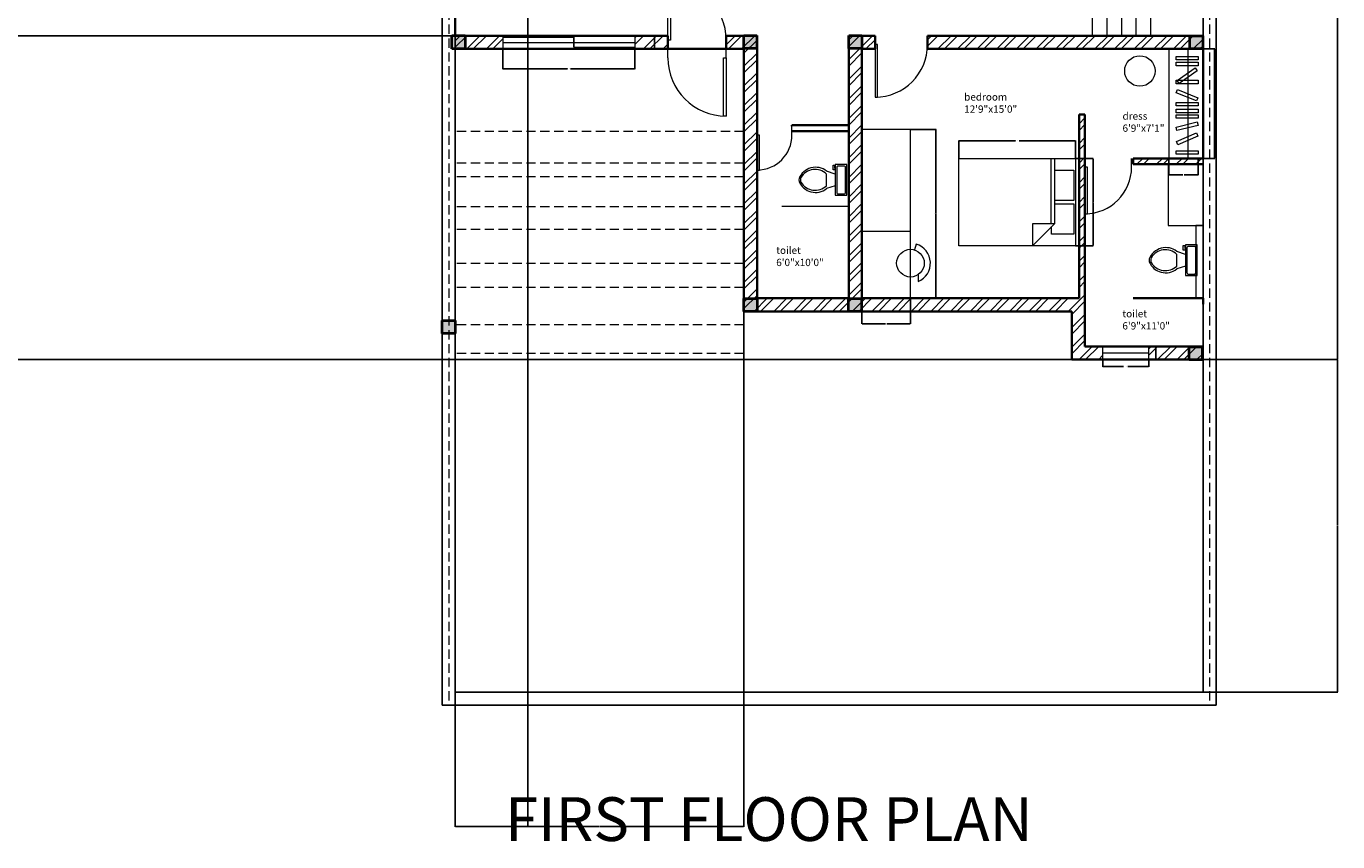
# Model space of a CAD drawing. Units: inches. Extents: x 19613 to 21413, y 12082 to 13202.
# Tile 7 of 9: x 20513 to 21413, y 12082 to 12641. Entities that reach past the tile are written whole.
import ezdxf

# ---------------------------------------------------------------- set-up
doc = ezdxf.new("R2010")
doc.units = ezdxf.units.IN
doc.linetypes.add('HIDDEN', pattern=[9.525, 6.35, -3.175])
for name, color, linetype, lineweight in [('A-ANNO-DIMS', 2, 'Continuous', 18), ('A-ANNO-TEXT', 7, 'Continuous', 30), ('A-AREA-IDEN', 7, 'Continuous', 18), ('A-COLS', 7, 'Continuous', 40), ('A-COLS-PATT', 6, 'Continuous', 13), ('A-DOOR', 3, 'Continuous', 18), ('A-FLOR-CASE', 9, 'Continuous', 18), ('A-FLOR-FIXT', 9, 'Continuous', 18), ('A-FLOR-HIDN', 8, 'HIDDEN', 13), ('A-FLOR-STRS', 7, 'Continuous', 18), ('A-FURN', 8, 'Continuous', 18), ('A-GLAZ', 4, 'Continuous', 18), ('A-WALL', 7, 'Continuous', 35), ('A-WALL-PATT', 252, 'Continuous', 13), ('C-PROP', 7, 'Continuous', 25), ('C-PROP-HIDN', 8, 'HIDDEN', 13)]:
    doc.layers.add(name, color=color, linetype=linetype, lineweight=lineweight)
doc.styles.get("Standard").update_dxf_attribs({"font": 'arial.ttf'})
doc.dimstyles.get("Standard").update_dxf_attribs({"dimtxt": 0.18, "dimasz": 0.18, "dimexe": 0.18, "dimexo": 0.0625, "dimgap": 0.09, "dimtad": 0, "dimtih": 1, "dimtoh": 1, "dimdec": 4, "dimzin": 0, "dimdsep": 46, "dimtxsty": 'Standard', "dimcen": 0.09, "dimadec": 0, "dimazin": 0, "dimtfac": 1, "dimtdec": 4, "dimtofl": 0, "dimtmove": 0, "dimatfit": 3, "dimfxl": 1, "dimtolj": 1, "dimtzin": 0, "dimarcsym": 0})

# ---------------------------------------------------------------- blocks, each defined once
blk = doc.blocks.new('Bed - Queen')
for p, q in [((0, -80.00003), (0, 0)), ((0, 0), (59.99999, 0)), ((59.99999, 0), (59.99999, -80.00003)), ((7.99999, -1.2), (28.79998, -1.2)), ((7.99999, -14.4), (7.99999, -1.2)), ((28.79998, -1.2), (28.79998, -14.4)), ((31.19999, -1.2), (51.99999, -1.2)), ((31.19999, -14.4), (31.19999, -1.2)), ((51.99999, -1.2), (51.99999, -16.4)), ((0, -14.4), (44.8, -14.4)), ((44.8, -16.8), (0, -16.8)), ((59.99999, -29.6), (44.8, -14.4)), ((44.8, -14.4), (44.8, -29.6)), ((51.99999, -16.4), (46.79936, -16.4)), ((44.8, -29.6), (59.99999, -29.6)), ((59.99999, -80.00003), (0, -80.00003))]:
    blk.add_line(p, q)
blk = doc.blocks.new('*U6')
for p, q in [((0, 0), (0, -6)), ((40, 0), (40, -6))]:
    blk.add_line(p, q)
blk.add_lwpolyline([(0, 0), (0, 40), (1.75, 40), (1.75, 0)], close=True)
blk.add_arc((0, 0), 40, 0, 90)
blk = doc.blocks.new('*U7')
for p, q in [((-40, 0), (-40, 6)), ((0, 0), (0, 6))]:
    blk.add_line(p, q)
blk.add_lwpolyline([(0, 0), (0, -40), (-1.75, -40), (-1.75, 0)], close=True)
blk.add_arc((0, 0), 40, 180, 270)
blk = doc.blocks.new('*U15')
for p, q in [((0, 0), (0, 6)), ((36, 0), (36, 6))]:
    blk.add_line(p, q)
blk.add_lwpolyline([(0, 0), (0, -36), (1.75, -36), (1.75, 0)], close=True)
blk.add_arc((0, 0), 36, 270, 0)
blk = doc.blocks.new('*U16')
for p, q in [((0, 0), (0, 6)), ((32, 0), (32, 6))]:
    blk.add_line(p, q)
blk.add_lwpolyline([(0, 0), (0, -32), (1.75, -32), (1.75, 0)], close=True)
blk.add_arc((0, 0), 32, 270, 0)
blk = doc.blocks.new('*U19')
for p, q in [((0, 0), (0, 6)), ((24, 0), (24, 6))]:
    blk.add_line(p, q)
blk.add_lwpolyline([(0, 0), (0, -24), (1.75, -24), (1.75, 0)], close=True)
blk.add_arc((0, 0), 24, 270, 0)
blk = doc.blocks.new('Toilet - top')
for p, q in [((-10, -8.5), (-8, -8.5)), ((-10, -9.5), (-10, -8.5)), ((-8, -8.5), (-8, -8)), ((-7, -8), (-7, -9.5)), ((-4, -8), (-6, -14)), ((4, -8), (6, -14)), ((9.5, -6), (9.5, -2)), ((-7, -9.5), (-10, -9.5)), ((4, -14), (-4, -14))]:
    blk.add_line(p, q)
blk.add_lwpolyline([(10.5, -8), (10.5, 0), (-10.5, 0), (-10.5, -8)], close=True)
for points in [[(-9.5, -2), (-9.5, -6)], [(8.5, -1), (-8.5, -1)], [(-8.5, -7), (8.5, -7)]]:
    blk.add_lwpolyline(points)
for centre, radius, start, end in [((-8.62, -1.88), 0.884, 81.8699, 188.1301), ((-8.62, -6.12), 0.884, 171.8699, 278.1301), ((8.62, -1.88), 0.884, 351.8699, 98.1301), ((8.62, -6.12), 0.884, 261.8699, 8.1301), ((3.52, -21.58), 12.17, 141.46911, 247.97143), ((4.2, -21.82), 11.33, 136.36773, 238.94682), ((-3.52, -21.58), 12.17, 292.02843, 38.53071), ((-4.2, -21.82), 11.33, 301.05301, 43.63209), ((0, -27.88), 4, 245.73182, 294.26817), ((0, -29), 4, 254.86053, 285.13947)]:
    blk.add_arc(centre, radius, start, end)
blk = doc.blocks.new('COL-9x9')
for p, q in [((0, 9), (9, 9)), ((0, 0), (0, 9)), ((9, 9), (9, 0)), ((9, 0), (0, 0))]:
    blk.add_line(p, q)
blk = doc.blocks.new('CLOSET-STRAIGHT-RAIL')
for p, q in [((0, 75), (0, 0)), ((12.99, 75), (12.99, 0))]:
    blk.add_line(p, q)
for points in [[(5.04, 69.91), (20.08, 69.91), (20.08, 67.47), (5.04, 67.47)], [(5.04, 65.98), (20.08, 65.98), (20.08, 63.54), (5.04, 63.54)], [(5.8, 53.4), (18.07, 62.1), (19.48, 60.12), (7.21, 51.41)], [(5.04, 53.51), (20.08, 53.51), (20.08, 51.08), (5.04, 51.08)], [(6.02, 47.16), (20, 41.61), (19.1, 39.35), (5.12, 44.9)], [(5.04, 38.4), (20.08, 38.4), (20.08, 35.96), (5.04, 35.96)], [(5.04, 33.62), (20.08, 33.62), (20.08, 31.19), (5.04, 31.19)], [(5.04, 29.93), (20.08, 29.93), (20.08, 27.49), (5.04, 27.49)], [(4.97, 21.36), (19.58, 24.94), (20.16, 22.57), (5.55, 18.99)], [(5.22, 11.51), (19.01, 17.5), (19.98, 15.27), (6.19, 9.28)], [(5.04, 5.23), (20.08, 5.23), (20.08, 2.79), (5.04, 2.79)]]:
    blk.add_lwpolyline(points, close=True)
blk = doc.blocks.new('WINDOW-LIVING-SLIDER')
for p, q in [((0, 9), (0, 0)), ((90.49, 9), (90.49, 0)), ((0, 8.08), (48.53, 8.08)), ((0, 4.5), (48.53, 4.5)), ((48.53, 4.5), (48.53, 8.08)), ((48.53, 8.08), (48.53, 1.28)), ((48.53, 1.28), (48.53, 4.5)), ((48.53, 4.5), (90.49, 4.5)), ((48.53, 1.28), (90.49, 1.28)), ((90.49, 6.86), (90.49, 4.5))]:
    blk.add_line(p, q)
blk = doc.blocks.new('WINDOW-BATH')
for p, q in [((0, 9), (0, 0)), ((31.63, 9), (31.63, 0)), ((0, 4.5), (31.63, 4.5))]:
    blk.add_line(p, q)
blk = doc.blocks.new('DESK-CHAIR-ROUND-LARGE')
for p, q in [((13.49, 25.67), (12.27, 21.68)), ((14.77, 4.71), (14.81, 0))]:
    blk.add_line(p, q)
blk.add_circle((9.49, 12.6), 9.49)
blk.add_circle((9.49, 12.6), 9.49)
blk.add_arc((9.49, 12.6), 13.67, 292.8714, 73.00761)
blk = doc.blocks.new('BEDROOM-DESK-WIDE')
for p, q in [((33.29, 115.88), (0, 115.88)), ((33.29, 0), (33.29, 115.88)), ((33.29, 45.86), (0, 45.86)), ((0, 0), (0, 0)), ((0, 0), (33.29, 0))]:
    blk.add_line(p, q)
blk = doc.blocks.new('STAIR-RETURN-FLIGHT')
for p, q in [((0, 169), (0, 133)), ((10, 169), (10, 133)), ((20, 169), (20, 133)), ((30, 169), (30, 133)), ((76, 169), (40, 169)), ((76, 169), (40, 169)), ((40, 169), (40, 0)), ((76, 169), (76, 133)), ((76, 169), (76, 133)), ((76, 133), (0, 133)), ((76, 123), (40, 123)), ((76, 113), (40, 113)), ((76, 103), (40, 103)), ((76, 93), (40, 93)), ((76, 83), (40, 83)), ((76, 73), (40, 73)), ((76, 63), (40, 63)), ((76, 31), (76, 67)), ((76, 53), (40, 53)), ((76, 36), (0, 36)), ((0, 36), (0, 0)), ((10, 36), (10, 0)), ((20, 36), (20, 0)), ((30, 36), (30, 0)), ((76, 43), (40, 43)), ((76, 0), (76, 36))]:
    blk.add_line(p, q)
blk = doc.blocks.new('*D41')
at = {"layer": 'A-ANNO-DIMS', "color": 0, "lineweight": -2, "transparency": 16777216}
for p, q in [((21153, 12550.29), (21153, 12562.41)), ((21153.18, 12562.23), (21191.69, 12562.23)), ((21232.82, 12562.23), (21194.3, 12562.23)), ((21233, 12550.29), (21233, 12562.41))]:
    blk.add_line(p, q, dxfattribs=at)
at = {"layer": 'A-ANNO-DIMS', "color": 0, "transparency": 16777216}
for points in [[(21153.18, 12562.26), (21153.18, 12562.2), (21153, 12562.23)], [(21232.82, 12562.26), (21232.82, 12562.2), (21233, 12562.23)]]:
    blk.add_solid(points, dxfattribs=at)
at = {"layer": 'Defpoints', "color": 0, "transparency": 16777216}
for p in [(21233, 12562.23), (21153, 12550.23), (21233, 12550.23)]:
    blk.add_point(p, dxfattribs=at)
at = {"layer": 'A-ANNO-DIMS', "color": 0, "transparency": 16777216, "insert": (21193, 12562.23), "char_height": 0.18, "attachment_point": 5}
blk.add_mtext('\\A1;QUEEN BED 80 TYP.', dxfattribs=at)
blk = doc.blocks.new('*D42')
at = {"layer": 'A-ANNO-DIMS', "color": 0, "lineweight": -2, "transparency": 16777216}
for p, q in [((21233.06, 12550.23), (21245.18, 12550.23)), ((21245, 12550.05), (21245, 12520.41)), ((21245, 12490.41), (21245, 12520.05)), ((21233.06, 12490.23), (21245.18, 12490.23))]:
    blk.add_line(p, q, dxfattribs=at)
at = {"layer": 'A-ANNO-DIMS', "color": 0, "transparency": 16777216}
for points in [[(21244.97, 12550.05), (21245.03, 12550.05), (21245, 12550.23)], [(21244.97, 12490.41), (21245.03, 12490.41), (21245, 12490.23)]]:
    blk.add_solid(points, dxfattribs=at)
at = {"layer": 'Defpoints', "color": 0, "transparency": 16777216}
for p in [(21233, 12550.23), (21233, 12490.23), (21245, 12490.23)]:
    blk.add_point(p, dxfattribs=at)
at = {"layer": 'A-ANNO-DIMS', "color": 0, "transparency": 16777216, "insert": (21245, 12520.23), "char_height": 0.18, "attachment_point": 5}
blk.add_mtext('\\A1;60 TYP.', dxfattribs=at)
blk = doc.blocks.new('*D57')
at = {"layer": 'A-ANNO-DIMS', "color": 0, "lineweight": -2, "transparency": 16777216}
for p, q in [((21317.16, 12625.28), (21328.52, 12625.28)), ((21328.34, 12625.1), (21328.34, 12587.96)), ((21328.34, 12550.46), (21328.34, 12587.6)), ((21317.16, 12550.28), (21328.52, 12550.28))]:
    blk.add_line(p, q, dxfattribs=at)
at = {"layer": 'A-ANNO-DIMS', "color": 0, "transparency": 16777216}
for points in [[(21328.31, 12625.1), (21328.37, 12625.1), (21328.34, 12625.28)], [(21328.31, 12550.46), (21328.37, 12550.46), (21328.34, 12550.28)]]:
    blk.add_solid(points, dxfattribs=at)
at = {"layer": 'Defpoints', "color": 0, "transparency": 16777216}
for p in [(21317.09, 12625.28), (21328.34, 12625.28), (21317.09, 12550.28)]:
    blk.add_point(p, dxfattribs=at)
at = {"layer": 'A-ANNO-DIMS', "color": 0, "transparency": 16777216, "insert": (21328.34, 12587.78), "char_height": 0.18, "attachment_point": 5}
blk.add_mtext('\\A1;RAIL 75 TYP.', dxfattribs=at)
blk = doc.blocks.new('*D58')
at = {"layer": 'A-ANNO-DIMS', "color": 0, "lineweight": -2, "transparency": 16777216}
for p, q in [((21296.94, 12550.22), (21296.94, 12538.85)), ((21317.09, 12550.22), (21317.09, 12538.85)), ((21297.12, 12539.03), (21306.49, 12539.03)), ((21316.91, 12539.03), (21307.55, 12539.03))]:
    blk.add_line(p, q, dxfattribs=at)
at = {"layer": 'A-ANNO-DIMS', "color": 0, "transparency": 16777216}
for points in [[(21297.12, 12539.06), (21297.12, 12539), (21296.94, 12539.03)], [(21316.91, 12539.06), (21316.91, 12539), (21317.09, 12539.03)]]:
    blk.add_solid(points, dxfattribs=at)
at = {"layer": 'Defpoints', "color": 0, "transparency": 16777216}
for p in [(21296.94, 12550.28), (21317.09, 12550.28), (21317.09, 12539.03)]:
    blk.add_point(p, dxfattribs=at)
at = {"layer": 'A-ANNO-DIMS', "color": 0, "transparency": 16777216, "insert": (21307.02, 12539.03), "char_height": 0.18, "attachment_point": 5}
blk.add_mtext('\\A1;20 TYP.', dxfattribs=at)
blk = doc.blocks.new('*D59')
at = {"layer": 'A-ANNO-DIMS', "color": 0, "lineweight": -2, "transparency": 16777216}
for p, q in [((20840.13, 12625.22), (20840.13, 12611.53)), ((20930.62, 12625.22), (20930.62, 12611.53)), ((20840.31, 12611.71), (20884.36, 12611.71)), ((20930.44, 12611.71), (20886.39, 12611.71))]:
    blk.add_line(p, q, dxfattribs=at)
at = {"layer": 'A-ANNO-DIMS', "color": 0, "transparency": 16777216}
for points in [[(20840.31, 12611.74), (20840.31, 12611.68), (20840.13, 12611.71)], [(20930.44, 12611.74), (20930.44, 12611.68), (20930.62, 12611.71)]]:
    blk.add_solid(points, dxfattribs=at)
at = {"layer": 'Defpoints', "color": 0, "transparency": 16777216}
for p in [(20840.13, 12625.28), (20930.62, 12625.28), (20930.62, 12611.71)]:
    blk.add_point(p, dxfattribs=at)
at = {"layer": 'A-ANNO-DIMS', "color": 0, "transparency": 16777216, "insert": (20885.38, 12611.71), "char_height": 0.18, "attachment_point": 5}
blk.add_mtext('\\A1;SLIDER 90 TYP.', dxfattribs=at)
blk = doc.blocks.new('*D60')
at = {"layer": 'A-ANNO-DIMS', "color": 0, "lineweight": -2, "transparency": 16777216}
for p, q in [((20930.68, 12634.28), (20944.37, 12634.28)), ((20944.19, 12634.1), (20944.19, 12629.96)), ((20930.68, 12625.28), (20944.37, 12625.28)), ((20944.19, 12625.46), (20944.19, 12629.6))]:
    blk.add_line(p, q, dxfattribs=at)
at = {"layer": 'A-ANNO-DIMS', "color": 0, "transparency": 16777216}
for points in [[(20944.16, 12634.1), (20944.22, 12634.1), (20944.19, 12634.28)], [(20944.16, 12625.46), (20944.22, 12625.46), (20944.19, 12625.28)]]:
    blk.add_solid(points, dxfattribs=at)
at = {"layer": 'Defpoints', "color": 0, "transparency": 16777216}
for p in [(20930.62, 12634.28), (20944.19, 12634.28), (20930.62, 12625.28)]:
    blk.add_point(p, dxfattribs=at)
at = {"layer": 'A-ANNO-DIMS', "color": 0, "transparency": 16777216, "insert": (20944.19, 12629.78), "char_height": 0.18, "attachment_point": 5}
blk.add_mtext('\\A1;9 TYP.', dxfattribs=at)
blk = doc.blocks.new('*D69')
at = {"layer": 'A-ANNO-DIMS', "color": 0, "lineweight": -2, "transparency": 16777216}
for p, q in [((21251.59, 12412.22), (21251.59, 12407.35)), ((21283.22, 12412.22), (21283.22, 12407.35)), ((21251.77, 12407.53), (21265.92, 12407.53)), ((21283.04, 12407.53), (21268.89, 12407.53))]:
    blk.add_line(p, q, dxfattribs=at)
at = {"layer": 'A-ANNO-DIMS', "color": 0, "transparency": 16777216}
for points in [[(21251.77, 12407.56), (21251.77, 12407.5), (21251.59, 12407.53)], [(21283.04, 12407.56), (21283.04, 12407.5), (21283.22, 12407.53)]]:
    blk.add_solid(points, dxfattribs=at)
at = {"layer": 'Defpoints', "color": 0, "transparency": 16777216}
for p in [(21251.59, 12412.28), (21283.22, 12412.28), (21251.59, 12407.53)]:
    blk.add_point(p, dxfattribs=at)
at = {"layer": 'A-ANNO-DIMS', "color": 0, "transparency": 16777216, "insert": (21267.41, 12407.53), "char_height": 0.18, "attachment_point": 5}
blk.add_mtext('\\A1;BATH WINDOW 32 TYP.', dxfattribs=at)
blk = doc.blocks.new('*D70')
at = {"layer": 'A-ANNO-DIMS', "color": 0, "lineweight": -2, "transparency": 16777216}
for p, q in [((21283.28, 12421.28), (21288.15, 12421.28)), ((21287.97, 12421.1), (21287.97, 12416.96)), ((21283.28, 12412.28), (21288.15, 12412.28)), ((21287.97, 12412.46), (21287.97, 12416.6))]:
    blk.add_line(p, q, dxfattribs=at)
at = {"layer": 'A-ANNO-DIMS', "color": 0, "transparency": 16777216}
for points in [[(21287.94, 12421.1), (21288, 12421.1), (21287.97, 12421.28)], [(21287.94, 12412.46), (21288, 12412.46), (21287.97, 12412.28)]]:
    blk.add_solid(points, dxfattribs=at)
at = {"layer": 'Defpoints', "color": 0, "transparency": 16777216}
for p in [(21283.22, 12421.28), (21283.22, 12412.28), (21287.97, 12412.28)]:
    blk.add_point(p, dxfattribs=at)
at = {"layer": 'A-ANNO-DIMS', "color": 0, "transparency": 16777216, "insert": (21287.97, 12416.78), "char_height": 0.18, "attachment_point": 5}
blk.add_mtext('\\A1;9 TYP.', dxfattribs=at)
blk = doc.blocks.new('*D73')
at = {"layer": 'A-ANNO-DIMS', "color": 0, "lineweight": -2, "transparency": 16777216}
for p, q in [((21119.79, 12570.15), (21137.29, 12570.15)), ((21137.11, 12569.97), (21137.11, 12512.4)), ((21137.11, 12454.46), (21137.11, 12512.03)), ((21119.79, 12454.28), (21137.29, 12454.28))]:
    blk.add_line(p, q, dxfattribs=at)
at = {"layer": 'A-ANNO-DIMS', "color": 0, "transparency": 16777216}
for points in [[(21137.08, 12569.97), (21137.14, 12569.97), (21137.11, 12570.15)], [(21137.08, 12454.46), (21137.14, 12454.46), (21137.11, 12454.28)]]:
    blk.add_solid(points, dxfattribs=at)
at = {"layer": 'Defpoints', "color": 0, "transparency": 16777216}
for p in [(21119.73, 12570.15), (21137.11, 12570.15), (21119.73, 12454.28)]:
    blk.add_point(p, dxfattribs=at)
at = {"layer": 'A-ANNO-DIMS', "color": 0, "transparency": 16777216, "insert": (21137.11, 12512.22), "char_height": 0.18, "attachment_point": 5}
blk.add_mtext('\\A1;DESK 116 TYP.', dxfattribs=at)
blk = doc.blocks.new('*D74')
at = {"layer": 'A-ANNO-DIMS', "color": 0, "lineweight": -2, "transparency": 16777216}
for p, q in [((21086.43, 12454.22), (21086.43, 12436.72)), ((21119.73, 12454.22), (21119.73, 12436.72)), ((21086.61, 12436.9), (21102.55, 12436.9)), ((21119.55, 12436.9), (21103.61, 12436.9))]:
    blk.add_line(p, q, dxfattribs=at)
at = {"layer": 'A-ANNO-DIMS', "color": 0, "transparency": 16777216}
for points in [[(21086.61, 12436.93), (21086.61, 12436.87), (21086.43, 12436.9)], [(21119.55, 12436.93), (21119.55, 12436.87), (21119.73, 12436.9)]]:
    blk.add_solid(points, dxfattribs=at)
at = {"layer": 'Defpoints', "color": 0, "transparency": 16777216}
for p in [(21086.43, 12454.28), (21119.73, 12454.28), (21119.73, 12436.9)]:
    blk.add_point(p, dxfattribs=at)
at = {"layer": 'A-ANNO-DIMS', "color": 0, "transparency": 16777216, "insert": (21103.08, 12436.9), "char_height": 0.18, "attachment_point": 5}
blk.add_mtext('\\A1;33 TYP.', dxfattribs=at)
blk = doc.blocks.new('*D87')
at = {"layer": 'A-ANNO-DIMS', "color": 0, "lineweight": -2, "transparency": 16777216}
for p, q in [((20218.76, 12982.28), (21412.86, 12982.28)), ((21412.68, 12982.1), (21412.68, 12697.46)), ((21412.68, 12412.46), (21412.68, 12697.1)), ((20218.76, 12412.28), (21412.86, 12412.28))]:
    blk.add_line(p, q, dxfattribs=at)
at = {"layer": 'A-ANNO-DIMS', "color": 0, "transparency": 16777216}
for points in [[(21412.65, 12982.1), (21412.71, 12982.1), (21412.68, 12982.28)], [(21412.65, 12412.46), (21412.71, 12412.46), (21412.68, 12412.28)]]:
    blk.add_solid(points, dxfattribs=at)
at = {"layer": 'Defpoints', "color": 0, "transparency": 16777216}
for p in [(20218.69, 12982.28), (21412.68, 12982.28), (20218.69, 12412.28)]:
    blk.add_point(p, dxfattribs=at)
at = {"layer": 'A-ANNO-DIMS', "color": 0, "transparency": 16777216, "insert": (21412.68, 12697.28), "char_height": 0.18, "attachment_point": 5}
blk.add_mtext('\\A1;570', dxfattribs=at)
blk = doc.blocks.new('*D88')
at = {"layer": 'A-ANNO-DIMS', "color": 0, "lineweight": -2, "transparency": 16777216}
for p, q in [((21320.5, 12412.28), (21412.86, 12412.28)), ((21412.68, 12412.1), (21412.68, 12298.46)), ((21412.68, 12184.46), (21412.68, 12298.1)), ((21320.5, 12184.28), (21412.86, 12184.28))]:
    blk.add_line(p, q, dxfattribs=at)
at = {"layer": 'A-ANNO-DIMS', "color": 0, "transparency": 16777216}
for points in [[(21412.65, 12412.1), (21412.71, 12412.1), (21412.68, 12412.28)], [(21412.65, 12184.46), (21412.71, 12184.46), (21412.68, 12184.28)]]:
    blk.add_solid(points, dxfattribs=at)
at = {"layer": 'Defpoints', "color": 0, "transparency": 16777216}
for p in [(21320.43, 12412.28), (21412.68, 12412.28), (21320.43, 12184.28)]:
    blk.add_point(p, dxfattribs=at)
at = {"layer": 'A-ANNO-DIMS', "color": 0, "transparency": 16777216, "insert": (21412.68, 12298.28), "char_height": 0.18, "attachment_point": 5}
blk.add_mtext('\\A1;228', dxfattribs=at)
blk = doc.blocks.new('*D89')
at = {"layer": 'A-ANNO-DIMS', "color": 0, "lineweight": -2, "transparency": 16777216}
for p, q in [((20807.37, 12808.28), (19613.26, 12808.28)), ((19613.44, 12808.1), (19613.44, 12721.46)), ((19613.44, 12634.46), (19613.44, 12721.1)), ((20807.37, 12634.28), (19613.26, 12634.28))]:
    blk.add_line(p, q, dxfattribs=at)
at = {"layer": 'A-ANNO-DIMS', "color": 0, "transparency": 16777216}
for points in [[(19613.41, 12808.1), (19613.47, 12808.1), (19613.44, 12808.28)], [(19613.41, 12634.46), (19613.47, 12634.46), (19613.44, 12634.28)]]:
    blk.add_solid(points, dxfattribs=at)
at = {"layer": 'Defpoints', "color": 0, "transparency": 16777216}
for p in [(19613.44, 12808.28), (20807.43, 12808.28), (20807.43, 12634.28)]:
    blk.add_point(p, dxfattribs=at)
at = {"layer": 'A-ANNO-DIMS', "color": 0, "transparency": 16777216, "insert": (19613.44, 12721.28), "char_height": 0.18, "attachment_point": 5}
blk.add_mtext('\\A1;174', dxfattribs=at)
blk = doc.blocks.new('*D99')
at = {"layer": 'A-ANNO-DIMS', "color": 0, "lineweight": -2, "transparency": 16777216}
for p, q in [((21320.5, 12982.28), (21412.86, 12982.28)), ((21412.68, 12982.1), (21412.68, 12697.46)), ((21412.68, 12412.46), (21412.68, 12697.1)), ((21320.5, 12412.28), (21412.86, 12412.28))]:
    blk.add_line(p, q, dxfattribs=at)
at = {"layer": 'A-ANNO-DIMS', "color": 0, "transparency": 16777216}
for points in [[(21412.65, 12982.1), (21412.71, 12982.1), (21412.68, 12982.28)], [(21412.65, 12412.46), (21412.71, 12412.46), (21412.68, 12412.28)]]:
    blk.add_solid(points, dxfattribs=at)
at = {"layer": 'Defpoints', "color": 0, "transparency": 16777216}
for p in [(21320.43, 12982.28), (21412.68, 12982.28), (21320.43, 12412.28)]:
    blk.add_point(p, dxfattribs=at)
at = {"layer": 'A-ANNO-DIMS', "color": 0, "transparency": 16777216, "insert": (21412.68, 12697.28), "char_height": 0.18, "attachment_point": 5}
blk.add_mtext('\\A1;570', dxfattribs=at)
blk = doc.blocks.new('*D100')
at = {"layer": 'A-ANNO-DIMS', "color": 0, "lineweight": -2, "transparency": 16777216}
for p, q in [((20807.43, 12973.22), (20807.43, 12091.85)), ((20857.28, 12973.22), (20857.28, 12091.85)), ((20807.61, 12092.03), (20831.96, 12092.03)), ((20857.1, 12092.03), (20832.75, 12092.03))]:
    blk.add_line(p, q, dxfattribs=at)
at = {"layer": 'A-ANNO-DIMS', "color": 0, "transparency": 16777216}
for points in [[(20807.61, 12092.06), (20807.61, 12092), (20807.43, 12092.03)], [(20857.1, 12092.06), (20857.1, 12092), (20857.28, 12092.03)]]:
    blk.add_solid(points, dxfattribs=at)
at = {"layer": 'Defpoints', "color": 0, "transparency": 16777216}
for p in [(20807.43, 12973.28), (20857.28, 12973.28), (20857.28, 12092.03)]:
    blk.add_point(p, dxfattribs=at)
at = {"layer": 'A-ANNO-DIMS', "color": 0, "transparency": 16777216, "insert": (20832.36, 12092.03), "char_height": 0.18, "attachment_point": 5}
blk.add_mtext('\\A1;49.85', dxfattribs=at)
blk = doc.blocks.new('*D104')
at = {"layer": 'A-ANNO-DIMS', "color": 0, "lineweight": -2, "transparency": 16777216}
for p, q in [((20807.43, 12625.22), (20807.43, 12091.85)), ((21005.43, 12625.22), (21005.43, 12091.85)), ((20807.61, 12092.03), (20906.15, 12092.03)), ((21005.25, 12092.03), (20906.71, 12092.03))]:
    blk.add_line(p, q, dxfattribs=at)
at = {"layer": 'A-ANNO-DIMS', "color": 0, "transparency": 16777216}
for points in [[(20807.61, 12092.06), (20807.61, 12092), (20807.43, 12092.03)], [(21005.25, 12092.06), (21005.25, 12092), (21005.43, 12092.03)]]:
    blk.add_solid(points, dxfattribs=at)
at = {"layer": 'Defpoints', "color": 0, "transparency": 16777216}
for p in [(20807.43, 12625.28), (21005.43, 12625.28), (21005.43, 12092.03)]:
    blk.add_point(p, dxfattribs=at)
at = {"layer": 'A-ANNO-DIMS', "color": 0, "transparency": 16777216, "insert": (20906.43, 12092.03), "char_height": 0.18, "attachment_point": 5}
blk.add_mtext('\\A1;198', dxfattribs=at)

msp = doc.modelspace()

# ---------------------------------------------------------------- hatches: boundary and pattern name
at = {"layer": 'A-COLS-PATT'}
h = msp.add_hatch(color=256, dxfattribs=at)
h.dxf.hatch_style = 1
h.paths.add_polyline_path([(20816.4328, 12982.279), (20807.4339, 12982.279), (20807.4339, 12973.279), (20816.4328, 12973.279)])
h.paths.add_polyline_path([(21084.4339, 12982.279), (21075.4339, 12982.279), (21075.4339, 12973.279), (21084.4339, 12973.279)])
h.paths.add_polyline_path([(21320.4339, 12982.279), (21311.4729, 12982.279), (21311.4729, 12973.279), (21320.4339, 12973.279)])
h.paths.add_polyline_path([(21320.3201, 12808.279), (21311.3201, 12808.279), (21311.3201, 12803.279), (21320.3201, 12803.279)])
h.paths.add_polyline_path([(21320.3201, 12812.279), (21311.3201, 12812.279), (21311.3201, 12808.279), (21320.3201, 12808.279)])
h.paths.add_polyline_path([(21320.3574, 12634.279), (21311.3574, 12634.279), (21311.3574, 12625.279), (21320.3574, 12625.279)])
h.paths.add_polyline_path([(21319.9035, 12421.1076), (21310.9035, 12421.1076), (21310.9035, 12412.279), (21319.9035, 12412.279)])
h.paths.add_polyline_path([(21086.1238, 12454.2407), (21077.1238, 12454.2407), (21077.1238, 12445.279), (21077.4339, 12445.279), (21086.1238, 12445.279)])
h.paths.add_polyline_path([(21014.4339, 12454.2407), (21005.4339, 12454.2407), (21005.4339, 12445.279), (21014.4339, 12445.279)])
h.paths.add_polyline_path([(21014.3637, 12634.279), (21005.3637, 12634.279), (21005.3637, 12625.5213), (21014.3637, 12625.5213)])
h.paths.add_polyline_path([(21086.4339, 12634.279), (21077.4339, 12634.279), (21077.4339, 12625.5213), (21086.4339, 12625.5213)])
h.paths.add_polyline_path([(20814.1423, 12634.279), (20807.4339, 12634.279), (20807.4339, 12625.4792), (20814.1423, 12625.4792)])
h.paths.add_polyline_path([(20807.4339, 12634.279), (20807.4339, 12634.4792), (20805.1423, 12634.4792), (20805.1423, 12625.4792), (20807.4339, 12625.4792)])
h.paths.add_polyline_path([(20807.4339, 12439.1296), (20802.9339, 12439.1296), (20802.9339, 12430.1296), (20807.4339, 12430.1296)])
h.paths.add_polyline_path([(20802.9339, 12439.1296), (20798.4339, 12439.1296), (20798.4339, 12430.1296), (20802.9339, 12430.1296)])
h.paths.add_polyline_path([(20813.4646, 12817.279), (20807.4339, 12817.279), (20807.4339, 12808.279), (20813.4646, 12808.279)])
h.paths.add_polyline_path([(20807.4339, 12817.279), (20804.4646, 12817.279), (20804.4646, 12808.279), (20807.4339, 12808.279)])
h.paths.add_polyline_path([(20896.8418, 12817.279), (20887.8418, 12817.279), (20887.8418, 12808.279), (20896.8418, 12808.279)])
h.paths.add_polyline_path([(21084.4339, 12817.279), (21075.4339, 12817.279), (21075.4339, 12808.279), (21084.4339, 12808.279)])
h.paths.add_polyline_path([(21201.8616, 12982.279), (21182.5788, 12982.279), (21182.5788, 12973.279), (21193.4339, 12973.279), (21201.8616, 12973.279), (21201.8616, 12976.279)])
at = {"layer": 'A-WALL-PATT'}
h = msp.add_hatch(dxfattribs=at)
h.set_pattern_fill('ANSI32', color=256)
h.paths.add_polyline_path([(20223.1937, 13118.279), (20218.6937, 13118.279), (19701.1937, 13118.279), (19701.1937, 13113.779), (20223.1937, 13113.779)])
h.paths.add_polyline_path([(19849.7315, 12982.279), (19799.9854, 12982.279), (19799.9854, 12973.279), (19849.7315, 12973.279)])
h.paths.add_polyline_path([(19755.5378, 12982.279), (19705.6937, 12982.279), (19705.6937, 12973.279), (19755.5378, 12973.279)])
h.paths.add_polyline_path([(20000.1054, 12982.279), (19950.0534, 12982.279), (19950.0534, 12974.1171), (19950.0534, 12973.279), (20000.1054, 12973.279)])
h.paths.add_polyline_path([(20049.4797, 12982.279), (20030.7476, 12982.279), (20030.7476, 12973.279), (20049.4797, 12973.279)])
h.paths.add_polyline_path([(20100.1214, 12982.279), (20080.8386, 12982.279), (20080.8386, 12973.279), (20100.1214, 12973.279), (20100.1214, 12976.279)])
h.paths.add_polyline_path([(20218.6937, 12982.279), (20167.6937, 12982.279), (20140.1214, 12982.279), (20140.1214, 12976.279, -0.01769781), (20140.0212, 12973.45), (20167.6937, 12973.279), (20176.6937, 12973.279), (20218.6937, 12973.279)])
h.paths.add_polyline_path([(19851.5503, 12814.279), (19851.5503, 12817.279), (19793.6937, 12817.279), (19789.6937, 12817.279), (19705.6937, 12817.279), (19705.6937, 12808.279), (19851.5503, 12808.279)])
h.paths.add_polyline_path([(19982.6937, 12973.279), (19973.6937, 12973.279), (19973.6937, 12817.279), (19887.5503, 12817.279), (19887.5503, 12808.279), (19973.6937, 12808.279), (19982.6937, 12808.279)])
h.paths.add_polyline_path([(20058.6937, 12850.5529), (19982.6937, 12850.5529), (19982.6937, 12846.5529), (20058.6937, 12846.5529)])
h.paths.add_polyline_path([(20095.6937, 12973.279), (20091.6937, 12973.279), (20091.6937, 12850.5529), (20087.6937, 12850.5529), (20087.6937, 12846.5529), (20095.6937, 12846.5529)])
h.paths.add_polyline_path([(20218.6937, 12808.279), (20140.8605, 12808.279), (20126.9413, 12808.279), (20126.9413, 12803.279), (20140.8605, 12803.279), (20218.6937, 12803.279)])
h.paths.add_polyline_path([(19738.3931, 12634.279), (19705.6937, 12634.279), (19705.6937, 12625.279), (19738.3931, 12625.279)])
h.paths.add_polyline_path([(19912.6937, 12634.279), (19903.6937, 12634.279), (19891.5503, 12634.279), (19891.5503, 12625.279), (19903.6937, 12625.279), (19903.6937, 12445.279), (19975.6937, 12445.279), (20128.6937, 12445.279), (20128.6937, 12412.279), (20149.8479, 12412.279), (20149.8479, 12421.279), (20137.6937, 12421.279), (20137.6937, 12454.279), (20137.6937, 12580.2801), (20133.6937, 12580.2801), (20133.6937, 12454.279), (19984.6937, 12454.279), (19984.6937, 12625.279), (19993.6937, 12625.279), (19993.6937, 12634.279), (19984.6937, 12634.279), (19975.6937, 12634.279), (19975.6937, 12454.279), (19912.6937, 12454.279)])
h.paths.add_polyline_path([(20218.6937, 12634.279), (20137.6937, 12634.279), (20029.6937, 12634.279), (20029.6937, 12625.279), (20137.6937, 12625.279), (20218.6937, 12625.279)])
h.paths.add_polyline_path([(21014.4339, 12634.279), (21005.4339, 12634.279), (20993.2905, 12634.279), (20993.2905, 12625.279), (21005.4339, 12625.279), (21005.4339, 12445.279), (21077.4339, 12445.279), (21230.4339, 12445.279), (21230.4339, 12412.279), (21251.5881, 12412.279), (21251.5881, 12421.279), (21239.4339, 12421.279), (21239.4339, 12454.279), (21239.4339, 12580.2801), (21235.4339, 12580.2801), (21235.4339, 12454.279), (21086.4339, 12454.279), (21086.4339, 12625.279), (21095.4339, 12625.279), (21095.4339, 12634.279), (21086.4339, 12634.279), (21077.4339, 12634.279), (21077.4339, 12454.279), (21014.4339, 12454.279)])
h.paths.add_polyline_path([(20840.1333, 12634.279), (20807.4339, 12634.279), (20807.4339, 12625.279), (20840.1333, 12625.279)])
h.paths.add_polyline_path([(20953.2905, 12631.279), (20953.2905, 12634.279), (20930.6216, 12634.279), (20930.6216, 12625.279), (20953.2905, 12625.279)])
h.paths.add_polyline_path([(21320.4339, 12634.279), (21239.4339, 12634.279), (21131.4339, 12634.279), (21131.4339, 12625.279), (21239.4339, 12625.279), (21320.4339, 12625.279)])
h.paths.add_polyline_path([(21084.4339, 12973.279), (21075.4339, 12973.279), (21075.4339, 12817.279), (20989.2905, 12817.279), (20989.2905, 12808.279), (21075.4339, 12808.279), (21084.4339, 12808.279)])
h.paths.add_polyline_path([(21142.1261, 12863.2893), (21084.4339, 12863.2893), (21084.4339, 12846.5529), (21142.1261, 12846.5529)])
h.paths.add_polyline_path([(21320.4339, 12808.279), (21242.6007, 12808.279), (21228.6815, 12808.279), (21228.6815, 12803.279), (21242.6007, 12803.279), (21320.4339, 12803.279)])
h.paths.add_polyline_path([(20857.278, 12982.279), (20807.4339, 12982.279), (20807.4339, 12973.279), (20857.278, 12973.279)])
h.paths.add_polyline_path([(20951.4717, 12982.279), (20901.7255, 12982.279), (20901.7255, 12973.279), (20951.4717, 12973.279)])
h.paths.add_polyline_path([(21101.8455, 12982.279), (21051.7936, 12982.279), (21051.7936, 12974.1171), (21051.7936, 12973.279), (21101.8455, 12973.279)])
h.paths.add_polyline_path([(21151.2199, 12982.279), (21132.4878, 12982.279), (21132.4878, 12973.279), (21151.2199, 12973.279)])
h.paths.add_polyline_path([(21201.8616, 12982.279), (21182.5788, 12982.279), (21182.5788, 12973.279), (21193.4339, 12973.279), (21201.8616, 12973.279), (21201.8616, 12976.279)])
h.paths.add_polyline_path([(21320.4339, 12982.279), (21269.4339, 12982.279), (21241.8616, 12982.279), (21241.8616, 12976.279, -0.01769781), (21241.7614, 12973.45), (21269.4339, 12973.279), (21278.4339, 12973.279), (21320.4339, 12973.279)])
h.paths.add_polyline_path([(20953.2905, 12817.279), (20895.4339, 12817.279), (20891.4339, 12817.279), (20807.4339, 12817.279), (20807.4339, 12808.279), (20953.2905, 12808.279)])
h.paths.add_polyline_path([(21197.4339, 12973.279), (21193.4339, 12973.279), (21193.4339, 12850.5529), (21197.4339, 12850.5529)])
h.paths.add_polyline_path([(21320.4339, 12550.279), (21272.5278, 12550.279), (21272.5278, 12546.279), (21320.4339, 12546.279)])
h.paths.add_polyline_path([(21320.4339, 12421.279), (21283.2222, 12421.279), (21283.2222, 12412.279), (21320.4339, 12412.279)])

# ---------------------------------------------------------------- linework, layer by layer
at = {"layer": 'A-FLOR-FIXT'}
for p, q in [((21296.4809, 12546.279), (21296.4809, 12504.2908)), ((21077.4339, 12517.279), (21031.583, 12517.279)), ((21077.4339, 12454.279), (21077.4339, 12517.279)), ((21296.4809, 12504.2908), (21320.4339, 12504.2908)), ((21320.4339, 12504.2908), (21315.4339, 12504.2908)), ((21315.4339, 12504.2908), (21315.4339, 12454.279))]:
    msp.add_line(p, q, dxfattribs=at)
at = {"layer": 'A-FLOR-HIDN'}
for p, q in [((21005.4339, 12568.5922), (20807.4339, 12568.5922)), ((21005.4339, 12546.9257), (20807.4339, 12546.9257)), ((21005.4339, 12537.5121), (20807.4339, 12537.5121)), ((21005.4339, 12517.0767), (20807.4339, 12517.0767)), ((21005.4339, 12501.5654), (20807.4339, 12501.5654)), ((21005.4339, 12478.224), (20807.4339, 12478.224)), ((21005.4339, 12461.658), (20807.4339, 12461.658)), ((21005.4339, 12445.279), (21005.4339, 12416.3791)), ((21005.4339, 12436.1373), (20807.4339, 12436.1373)), ((21005.4339, 12416.3791), (20807.4339, 12416.3791))]:
    msp.add_line(p, q, dxfattribs=at)
at = {"layer": 'A-FURN'}
msp.add_circle((21277.1089, 12610.1834), 10.4264, dxfattribs=at)
at = {"layer": 'A-WALL'}
for p, q in [((20807.4339, 12808.279), (20807.4339, 12634.279)), ((20807.4339, 12634.279), (20953.2905, 12634.279)), ((20807.4339, 12634.279), (20848.157, 12634.279)), ((20953.2905, 12634.279), (20953.2905, 12625.279)), ((21005.4339, 12634.279), (20993.2905, 12634.279)), ((20993.2905, 12634.279), (20993.2905, 12625.279)), ((21005.4339, 12634.279), (21014.4339, 12634.279)), ((21014.4339, 12454.279), (21014.4339, 12634.279)), ((21077.4339, 12634.279), (21077.4339, 12454.279)), ((21077.4339, 12634.279), (21086.4339, 12634.279)), ((21095.4339, 12634.279), (21086.4339, 12634.279)), ((21086.4339, 12634.279), (21095.4339, 12634.279)), ((21095.4339, 12634.279), (21095.4339, 12625.279)), ((21239.4339, 12634.279), (21131.4339, 12634.279)), ((21131.4339, 12625.279), (21131.4339, 12634.279)), ((21320.4339, 12634.279), (21239.4339, 12634.279)), ((21320.4339, 12634.279), (21320.4339, 12550.279)), ((20953.2905, 12625.279), (20807.4339, 12625.279)), ((20953.2905, 12625.279), (21005.4339, 12625.279)), ((20993.2905, 12625.279), (21005.4339, 12625.279)), ((21005.4339, 12445.279), (21005.4339, 12625.279)), ((21095.4339, 12625.279), (21086.4339, 12625.279)), ((21086.4339, 12625.279), (21086.4339, 12454.279)), ((21239.4339, 12625.279), (21131.4339, 12625.279)), ((21320.4339, 12625.279), (21239.4339, 12625.279)), ((21235.4339, 12454.279), (21235.4339, 12580.2801)), ((21235.4339, 12580.2801), (21239.4339, 12580.2801)), ((21239.4339, 12454.279), (21239.4339, 12580.2801)), ((21077.4339, 12572.9433), (21038.4339, 12572.9433)), ((21038.4339, 12572.2779), (21038.4339, 12572.9433)), ((21038.4339, 12568.9433), (21077.4339, 12568.9433)), ((21320.4339, 12550.279), (21272.5278, 12550.279)), ((21272.5278, 12550.279), (21272.5278, 12546.279)), ((21272.5278, 12546.279), (21320.4339, 12546.279)), ((21077.4339, 12454.279), (21014.4339, 12454.279)), ((21086.4339, 12454.279), (21235.4339, 12454.279)), ((21239.4339, 12454.279), (21239.4339, 12421.279)), ((21239.4339, 12421.279), (21239.4339, 12454.279)), ((21239.4339, 12421.279), (21239.4339, 12454.279)), ((21272.5278, 12454.279), (21320.4339, 12454.279)), ((21320.4339, 12454.279), (21320.4339, 12450.279)), ((21077.4339, 12445.279), (21005.4339, 12445.279)), ((21077.4339, 12445.279), (21230.4339, 12445.279)), ((21230.4339, 12412.279), (21230.4339, 12445.279)), ((21239.4339, 12421.279), (21320.4339, 12421.279)), ((21230.4339, 12412.279), (21320.4339, 12412.279))]:
    msp.add_line(p, q, dxfattribs=at)
at = {"layer": 'C-PROP'}
for p, q in [((20798.4339, 12175.279), (20798.4339, 13118.279)), ((21329.4339, 13118.279), (21329.4339, 12175.279)), ((20807.4339, 13109.279), (20807.4339, 12184.279)), ((21320.4339, 13109.279), (21320.4339, 12184.279)), ((21320.4339, 12184.279), (21320.4339, 12412.279)), ((20798.4339, 12175.279), (20798.4339, 12184.279)), ((20807.4339, 12184.279), (21320.4339, 12184.279)), ((21329.4339, 12175.279), (20798.4339, 12175.279))]:
    msp.add_line(p, q, dxfattribs=at)
at = {"layer": 'C-PROP-HIDN'}
for p, q in [((20802.9339, 13118.279), (20802.9339, 12175.279)), ((21324.9339, 13118.279), (21324.9339, 12175.279))]:
    msp.add_line(p, q, dxfattribs=at)

# ---------------------------------------------------------------- block references
at = {"layer": 'A-COLS', "rotation": 180}
for p in [(20814.1427, 12634.4792), (21014.3641, 12634.5213), (21086.4343, 12634.5213), (21320.3578, 12634.279), (21014.4343, 12454.2407), (21086.1242, 12454.2407), (20807.4343, 12439.1296), (21319.9039, 12421.1076)]:
    msp.add_blockref('COL-9x9', p, dxfattribs=at)
at = {"layer": 'A-DOOR'}
for name, p in [('*U6', (20953.2905, 12631.279)), ('*U15', (21095.4339, 12628.279)), ('*U7', (20993.2905, 12619.279)), ('*U19', (21014.4339, 12566.2779)), ('*U16', (21239.4339, 12544.279))]:
    msp.add_blockref(name, p, dxfattribs=at)
at = {"layer": 'A-FLOR-CASE'}
msp.add_blockref('CLOSET-STRAIGHT-RAIL', (21296.9372, 12550.279), dxfattribs=at)
at = {"layer": 'A-FLOR-FIXT', "rotation": 270}
for p in [(21076.1377, 12535.5118), (21316.425, 12480.4128)]:
    msp.add_blockref('Toilet - top', p, dxfattribs=at)
at = {"layer": 'A-FLOR-STRS'}
msp.add_blockref('STAIR-RETURN-FLIGHT', (21244.4342, 12634.279), dxfattribs=at)
at = {"layer": 'A-FURN'}
for name, p in [('BEDROOM-DESK-WIDE', (21086.4342, 12454.279)), ('DESK-CHAIR-ROUND-LARGE', (21110.2322, 12465.795))]:
    msp.add_blockref(name, p, dxfattribs=at)
at = {"layer": 'A-FURN', "rotation": 270.0000000000108}
msp.add_blockref('Bed - Queen', (21232.9962, 12550.2322), dxfattribs=at)
at = {"layer": 'A-GLAZ'}
msp.add_blockref('WINDOW-LIVING-SLIDER', (20840.1332, 12625.279), dxfattribs=at)
at = {"layer": 'A-GLAZ', "rotation": 180}
msp.add_blockref('WINDOW-BATH', (21283.2221, 12421.279), dxfattribs=at)

# ---------------------------------------------------------------- texts
at = {"layer": 'A-ANNO-TEXT', "insert": (20841.6266, 12112.127), "char_height": 30, "attachment_point": 1}
msp.add_mtext_dynamic_manual_height_columns('FIRST FLOOR PLAN', width=510.437427, gutter_width=12.5, heights=[0], dxfattribs=at)
at = {"layer": 'A-AREA-IDEN', "char_height": 5, "attachment_point": 1}
for s, insert in [('bedroom\\P12\'9"x15\'0"', (21156.5773, 12594.8852)), ('dress\\P6\'9"x7\'1"', (21265.2118, 12581.7993)), ('toilet\\P6\'0"x10\'0"', (21027.6328, 12489.7229)), ('toilet\\P6\'9"x11\'0"', (21265.1363, 12446.2378))]:
    msp.add_mtext_dynamic_manual_height_columns(s, width=19.652904, gutter_width=12.5, heights=[0], dxfattribs=dict(at, insert=insert))

# ---------------------------------------------------------------- dimensions: what is measured, and where the dimension line sits
at = {"layer": 'A-ANNO-DIMS'}
for base, p1, p2, picture, middle in [((21412.6839, 12982.279), (20218.6937, 12412.279), (20218.6937, 12982.279), '*D87', (21412.6839, 12697.279)), ((21412.6839, 12982.279), (21320.4339, 12412.279), (21320.4339, 12982.279), '*D99', (21412.6839, 12697.279)), ((19613.4437, 12808.279), (20807.4339, 12634.279), (20807.4339, 12808.279), '*D89', (19613.4437, 12721.279)), ((21412.6839, 12412.279), (21320.4339, 12184.279), (21320.4339, 12412.279), '*D88', (21412.6839, 12298.279))]:
    dim = msp.add_linear_dim(base=base, p1=p1, p2=p2, angle=90, dimstyle='Standard', override={"dimdec": 0, "dimlfac": 1, "dimrnd": 0, "dimzin": 0, "dimdsep": 46, "dimlunit": 2}, dxfattribs=at)
    dim.commit()
    dim.dimension.update_dxf_attribs({"geometry": picture, "text_midpoint": middle})
for base, p1, p2, override, picture, middle in [((20857.278, 12092.029), (20807.4328, 12973.279), (20857.278, 12973.279), {"dimdec": 2, "dimlfac": 1, "dimrnd": 0, "dimzin": 0, "dimdsep": 46, "dimlunit": 2}, '*D100', (20832.3554, 12092.029)), ((21005.4339, 12092.029), (20807.4339, 12625.279), (21005.4339, 12625.279), {"dimdec": 0, "dimlfac": 1, "dimrnd": 0, "dimzin": 0, "dimdsep": 46, "dimlunit": 2}, '*D104', (20906.4339, 12092.029))]:
    dim = msp.add_linear_dim(base=base, p1=p1, p2=p2, dimstyle='Standard', override=override, dxfattribs=at)
    dim.commit()
    dim.dimension.update_dxf_attribs({"geometry": picture, "text_midpoint": middle})
for base, p1, p2, angle, text, picture, middle in [((20944.1949, 12634.279), (20930.6216, 12625.279), (20930.6216, 12634.279), 90, '<> TYP.', '*D60', (20944.1949, 12629.779)), ((21328.3443, 12625.279), (21317.0943, 12550.279), (21317.0943, 12625.279), 90, 'RAIL <> TYP.', '*D57', (21328.3443, 12587.779)), ((21137.1064, 12570.1541), (21119.7251, 12454.279), (21119.7251, 12570.1541), 90, 'DESK <> TYP.', '*D73', (21137.1064, 12512.2165)), ((21232.9962, 12562.2322), (21152.9961, 12550.2322), (21232.9962, 12550.2322), 0, 'QUEEN BED <> TYP.', '*D41', (21192.9961, 12562.2322)), ((21244.9962, 12490.2322), (21232.9962, 12550.2322), (21232.9962, 12490.2322), 270, '<> TYP.', '*D42', (21244.9962, 12520.2322)), ((21287.9673, 12412.279), (21283.2222, 12421.279), (21283.2222, 12412.279), 270, '<> TYP.', '*D70', (21287.9673, 12416.779)), ((21251.5881, 12407.5339), (21283.2222, 12412.279), (21251.5881, 12412.279), 180, 'BATH WINDOW <> TYP.', '*D69', (21267.4052, 12407.5339))]:
    dim = msp.add_linear_dim(base=base, p1=p1, p2=p2, angle=angle, text=text, dimstyle='Standard', override={"dimdec": 0, "dimlfac": 1, "dimrnd": 0, "dimzin": 0, "dimdsep": 46, "dimlunit": 2}, dxfattribs=at)
    dim.commit()
    dim.dimension.update_dxf_attribs({"geometry": picture, "text_midpoint": middle})
for base, p1, p2, text, picture, middle in [((20930.6216, 12611.7057), (20840.1333, 12625.279), (20930.6216, 12625.279), 'SLIDER <> TYP.', '*D59', (20885.3775, 12611.7057)), ((21317.0943, 12539.029), (21296.9374, 12550.279), (21317.0943, 12550.279), '<> TYP.', '*D58', (21307.0159, 12539.029)), ((21119.7251, 12436.8977), (21086.4339, 12454.279), (21119.7251, 12454.279), '<> TYP.', '*D74', (21103.0795, 12436.8977))]:
    dim = msp.add_linear_dim(base=base, p1=p1, p2=p2, text=text, dimstyle='Standard', override={"dimdec": 0, "dimlfac": 1, "dimrnd": 0, "dimzin": 0, "dimdsep": 46, "dimlunit": 2}, dxfattribs=at)
    dim.commit()
    dim.dimension.update_dxf_attribs({"geometry": picture, "text_midpoint": middle})

doc.saveas('drawing.dxf')
